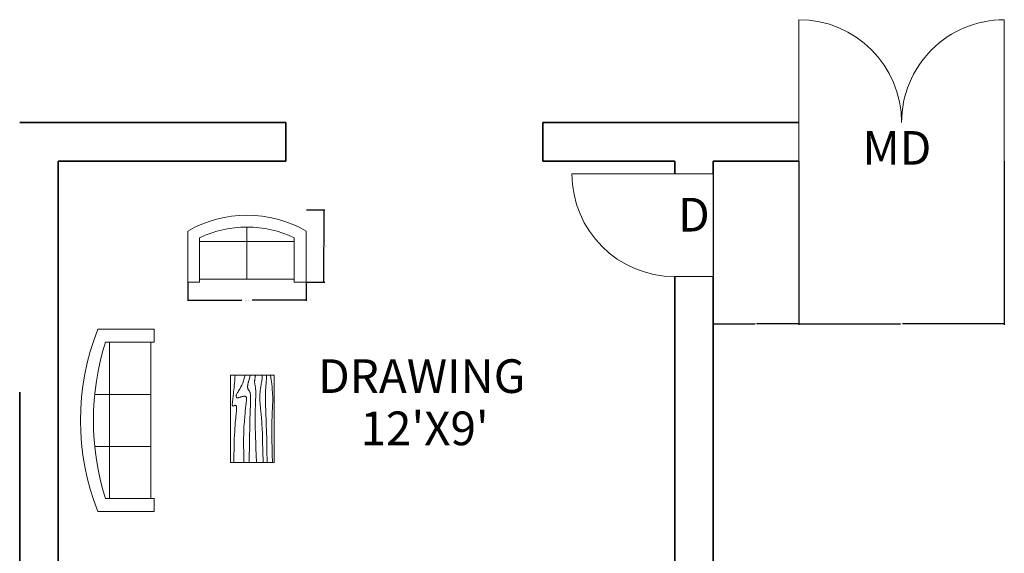
# Model space of a CAD drawing. Units: feet. Extents: x 2219 to 3039, y 1768 to 2369.
# Tile 5 of 16: x 2601 to 2831, y 2021 to 2146. Entities that reach past the tile are written whole.
import ezdxf

# ---------------------------------------------------------------- set-up
doc = ezdxf.new("R2010")
doc.units = ezdxf.units.FT
for name, color, linetype, lineweight in [('A-ANNO-DIMS', 2, 'Continuous', 18), ('A-ANNO-TEXT', 7, 'Continuous', 18), ('A-AREA-IDEN', 7, 'Continuous', 18), ('A-DOOR', 4, 'Continuous', 20), ('A-FURN', 8, 'Continuous', 18), ('A-WALL', 7, 'Continuous', 35)]:
    doc.layers.add(name, color=color, linetype=linetype, lineweight=lineweight)
doc.styles.get("Standard").update_dxf_attribs({"font": 'arial.ttf'})
doc.dimstyles.get("Standard").update_dxf_attribs({"dimtxt": 0.18, "dimasz": 0.18, "dimexe": 0.18, "dimexo": 0.0625, "dimgap": 0.09, "dimtad": 0, "dimtih": 1, "dimtoh": 1, "dimdec": 4, "dimzin": 0, "dimdsep": 46, "dimtxsty": 'Standard', "dimcen": 0.09, "dimadec": 0, "dimazin": 0, "dimtfac": 1, "dimtdec": 4, "dimtofl": 0, "dimtmove": 0, "dimatfit": 3, "dimfxl": 1, "dimtolj": 1, "dimtzin": 0, "dimarcsym": 0})

# ---------------------------------------------------------------- blocks, each defined once
blk = doc.blocks.new('Sofa - Roundback 7 ft.')
for p, q in [((-12.00002, -32.4421), (-12.00003, -6.5971)), ((11.99997, -32.4421), (11.99998, -6.5971)), ((-36.000027, -34), (-36.000027, -11.4696)), ((-35.999844, -13.3819), (35.9998, -13.3819)), ((35.99998, -34), (35.99998, -11.4696)), ((-36.000027, -32.4421), (35.99998, -32.4421))]:
    blk.add_line(p, q)
for points in [[(-36.000027, -34), (-42.000027, -34), (-42.000027, -8)], [(41.99998, -8), (41.99998, -34), (35.99998, -34)]]:
    blk.add_lwpolyline(points)
for centre, radius, start, end in [((0, -114.25), 114.25, 68.43141, 111.5686), ((-0.00001, -127.1968), 121.1968, 72.72033, 107.2797)]:
    blk.add_arc(centre, radius, start, end)
blk = doc.blocks.new('Sofa - Roundback Loveseat 5 ft.')
for p, q in [((0, -32.44198), (0, -5.99998)), ((-24, -33.99998), (-24, -11.46958)), ((-23.9998, -13.38178), (23.99986, -13.38178)), ((24.00004, -33.99998), (24.00004, -11.46958)), ((-24, -32.44198), (24.00004, -32.44198))]:
    blk.add_line(p, q)
for points in [[(-24, -33.99998), (-30, -33.99998), (-30, -7.99998)], [(30.00004, -7.99998), (30.00004, -33.99998), (24.00004, -33.99998)]]:
    blk.add_lwpolyline(points)
for centre, radius, start, end in [((0, -60.24998), 60.24998, 60.13715, 119.8628), ((0, -61.38438), 55.38444, 64.32083, 115.6792)]:
    blk.add_arc(centre, radius, start, end)
blk = doc.blocks.new('Table - Rectangular Woodgrain 60 x 30 in.')
for p, q in [((0, 0), (0, -30)), ((60, 0), (0, 0)), ((60, -30), (60, 0)), ((0, -30), (60, -30))]:
    blk.add_line(p, q)
for points in [[(0, -2.4), (4.8155, -2.418), (9.0302, -2.4688), (12.709, -2.5477), (15.9167, -2.65), (18.7181, -2.7711), (21.1781, -2.9063), (23.3616, -3.0508), (25.3333, -3.2), (27.1477, -3.3495), (28.8172, -3.4958), (30.3437, -3.636), (31.7291, -3.7667), (32.9756, -3.8849), (34.0849, -3.9875), (35.059, -4.0714), (35.9, -4.1334), (36.6114, -4.1711), (37.2041, -4.1854), (37.6906, -4.1779), (38.0833, -4.15), (38.3948, -4.1034), (38.6375, -4.0396), (38.8239, -3.9602), (38.9666, -3.8667), (39.0764, -3.7608), (39.1573, -3.6448), (39.2116, -3.521), (39.2416, -3.3917), (39.2498, -3.2593), (39.2385, -3.1261), (39.21, -2.9944), (39.1666, -2.8667), (39.111, -2.7447), (39.0468, -2.6281), (38.978, -2.5163), (38.9083, -2.4083), (38.8418, -2.3035), (38.7823, -2.201), (38.7337, -2.1001), (38.7, -2), (38.6844, -1.9003), (38.6875, -1.8021), (38.7094, -1.707), (38.75, -1.6167), (38.8094, -1.5326), (38.8875, -1.4563), (38.9844, -1.3893), (39.1, -1.3333), (39.2351, -1.2896), (39.3937, -1.2583), (39.5804, -1.2396), (39.8, -1.2333), (40.057, -1.2396), (40.3562, -1.2583), (40.7023, -1.2896), (41.1, -1.3333), (41.5547, -1.3895), (42.0755, -1.4573), (42.6721, -1.5361), (43.3542, -1.625), (44.1316, -1.7233), (45.014, -1.8302), (46.0114, -1.9449), (47.1333, -2.0667), (48.3862, -2.1947), (49.7625, -2.3281), (51.2513, -2.4663), (52.8416, -2.6083), (54.5226, -2.7535), (56.2833, -2.9011), (58.1127, -3.0501), (60, -3.2)], [(0, -9.2), (6.5759, -9.0858), (11.9385, -9.0365), (16.2527, -9.0418), (19.6833, -9.0917), (22.3952, -9.1759), (24.5531, -9.2844), (26.322, -9.4069), (27.8666, -9.5333), (29.3241, -9.6553), (30.7203, -9.7719), (32.0532, -9.8837), (33.3208, -9.9917), (34.5213, -10.0965), (35.6526, -10.199), (36.7128, -10.2999), (37.7, -10.4), (38.6129, -10.4996), (39.4531, -10.5969), (40.223, -10.6895), (40.925, -10.775), (41.5613, -10.8512), (42.1344, -10.9156), (42.6465, -10.966), (43.1, -11), (43.4976, -11.0158), (43.8437, -11.0136), (44.143, -10.9942), (44.4, -10.9583), (44.6195, -10.9069), (44.8062, -10.8406), (44.9648, -10.7603), (45.1, -10.6667), (45.2155, -10.5598), (45.3114, -10.4365), (45.3871, -10.2929), (45.4416, -10.125), (45.4743, -9.929), (45.4844, -9.7011), (45.4709, -9.4371), (45.4333, -9.1333), (45.3716, -8.7883), (45.2896, -8.4104), (45.1919, -8.0107), (45.0833, -7.6), (44.9685, -7.1893), (44.8521, -6.7896), (44.7388, -6.4117), (44.6333, -6.0667), (44.54, -5.7628), (44.4614, -5.4979), (44.4001, -5.2675), (44.3583, -5.0667), (44.3384, -4.8909), (44.3427, -4.7354), (44.3736, -4.5956), (44.4333, -4.4667), (44.5236, -4.3453), (44.6427, -4.2333), (44.7884, -4.1339), (44.9583, -4.05), (45.1501, -3.9849), (45.3614, -3.9417), (45.59, -3.9234), (45.8333, -3.9333), (46.0915, -3.9749), (46.3734, -4.0531), (46.6906, -4.1736), (47.0542, -4.3417), (47.4756, -4.5629), (47.9661, -4.8427), (48.5372, -5.1866), (49.2, -5.6), (49.9676, -6.0844), (50.8594, -6.625), (51.8965, -7.2031), (53.1, -7.8), (54.491, -8.3969), (56.0906, -8.975), (57.9199, -9.5156), (60, -10)], [(0, -12.8), (5.1847, -12.9322), (9.6213, -13.0323), (13.3963, -13.1059), (16.5958, -13.1583), (19.3063, -13.1952), (21.614, -13.2219), (23.6054, -13.2439), (25.3666, -13.2667), (26.9728, -13.2947), (28.4531, -13.3281), (29.8256, -13.3663), (31.1083, -13.4083), (32.3191, -13.4535), (33.476, -13.501), (34.597, -13.5501), (35.7, -13.6), (36.7984, -13.6497), (37.8875, -13.6979), (38.9578, -13.743), (40, -13.7833), (41.0047, -13.8174), (41.9625, -13.8438), (42.864, -13.8607), (43.7, -13.8667), (44.4631, -13.8604), (45.1552, -13.8417), (45.7801, -13.8104), (46.3416, -13.7667), (46.8439, -13.7104), (47.2906, -13.6417), (47.6858, -13.5604), (48.0333, -13.4667), (48.3375, -13.3608), (48.6042, -13.2448), (48.8396, -13.121), (49.05, -12.9917), (49.2417, -12.8593), (49.4208, -12.7261), (49.5937, -12.5944), (49.7667, -12.4667), (49.9452, -12.3451), (50.1323, -12.2313), (50.3303, -12.1268), (50.5416, -12.0333), (50.7686, -11.9524), (51.0135, -11.8854), (51.2788, -11.8341), (51.5666, -11.8), (51.8785, -11.7843), (52.2116, -11.7865), (52.562, -11.8059), (52.926, -11.8417), (53.2998, -11.8931), (53.6795, -11.9594), (54.0614, -12.0397), (54.4416, -12.1333), (54.8223, -12.2401), (55.2293, -12.3625), (55.6942, -12.5037), (56.2489, -12.6667), (56.9251, -12.8547), (57.7545, -13.0708), (58.7689, -13.3182), (60, -13.6)], [(0, -18), (5.124, -17.7273), (9.6609, -17.5057), (13.6705, -17.3303), (17.2125, -17.1958), (20.3467, -17.0973), (23.1328, -17.0297), (25.6307, -16.9878), (27.9, -16.9667), (29.9928, -16.9617), (31.9302, -16.9703), (33.7254, -16.9907), (35.3917, -17.0208), (36.9423, -17.0588), (38.3906, -17.1026), (39.7499, -17.1503), (41.0333, -17.2), (42.2519, -17.2496), (43.4073, -17.2969), (44.4986, -17.3395), (45.525, -17.375), (46.4858, -17.4012), (47.3802, -17.4156), (48.2074, -17.416), (48.9667, -17.4), (49.6583, -17.3662), (50.2872, -17.3167), (50.8595, -17.2547), (51.3812, -17.1833), (51.8584, -17.1057), (52.2971, -17.025), (52.7034, -16.9443), (53.0833, -16.8667), (53.443, -16.7951), (53.789, -16.7313), (54.128, -16.6768), (54.4666, -16.6334), (54.8115, -16.6024), (55.1693, -16.5854), (55.5465, -16.5841), (55.95, -16.6), (56.3828, -16.6337), (56.8346, -16.6823), (57.2915, -16.7418), (57.7396, -16.8084), (58.165, -16.878), (58.5539, -16.9469), (58.8924, -17.0111), (59.1666, -17.0667), (59.3679, -17.1107), (59.5078, -17.1438), (59.6032, -17.1675), (59.6708, -17.1833), (59.7275, -17.193), (59.7901, -17.1979), (59.8753, -17.1998), (60, -17.2)], [(0, -22.4), (8.0098, -22.2501), (14.4094, -22.1011), (19.4168, -21.9535), (23.25, -21.8083), (26.1269, -21.6663), (28.2656, -21.5281), (29.884, -21.3947), (31.2, -21.2667), (32.3967, -21.1448), (33.5172, -21.0292), (34.5697, -20.9198), (35.5625, -20.8167), (36.5037, -20.7198), (37.4015, -20.6292), (38.2642, -20.5448), (39.1, -20.4667), (39.9164, -20.3951), (40.7187, -20.3313), (41.5117, -20.2768), (42.3, -20.2333), (43.0883, -20.2024), (43.8812, -20.1854), (44.6836, -20.1841), (45.5, -20.2), (46.3328, -20.234), (47.1747, -20.2844), (48.0163, -20.3488), (48.8479, -20.425), (49.66, -20.5106), (50.4429, -20.6031), (51.1872, -20.7004), (51.8833, -20.8), (52.5246, -20.8999), (53.1166, -20.9995), (53.6681, -21.0983), (54.1875, -21.1958), (54.6834, -21.2919), (55.1646, -21.3859), (55.6394, -21.4777), (56.1167, -21.5667), (56.6028, -21.6515), (57.0961, -21.7266), (57.5929, -21.7852), (58.0896, -21.8208), (58.5823, -21.8268), (59.0674, -21.7964), (59.5412, -21.723), (60, -21.6)], [(0, -25.2), (8.6355, -25.0504), (15.7026, -24.9031), (21.4049, -24.7606), (25.9458, -24.625), (29.529, -24.4988), (32.3578, -24.3844), (34.6359, -24.284), (36.5667, -24.2), (38.3213, -24.1341), (39.9417, -24.0854), (41.437, -24.0523), (42.8167, -24.0333), (44.0901, -24.0268), (45.2667, -24.0313), (46.3557, -24.0451), (47.3667, -24.0667), (48.309, -24.0947), (49.1928, -24.1287), (50.0284, -24.168), (50.826, -24.2125), (51.5959, -24.2617), (52.3483, -24.3151), (53.0935, -24.3725), (53.8417, -24.4334), (54.6009, -24.497), (55.3699, -24.561), (56.1454, -24.6226), (56.9239, -24.6792), (57.7021, -24.7279), (58.4764, -24.7662), (59.2435, -24.7911), (60, -24.8)], [(0, -28.8), (5.6867, -28.6681), (10.45, -28.5698), (14.407, -28.5012), (17.675, -28.4584), (20.3711, -28.4374), (22.6125, -28.4344), (24.5164, -28.4455), (26.2, -28.4667), (27.762, -28.4947), (29.2276, -28.5281), (30.6033, -28.5663), (31.8958, -28.6084), (33.1118, -28.6535), (34.2578, -28.7011), (35.3405, -28.7501), (36.3666, -28.8), (37.3443, -28.8497), (38.288, -28.8974), (39.2137, -28.9412), (40.1375, -28.9792), (41.0753, -29.0093), (42.0432, -29.0297), (43.0572, -29.0384), (44.1333, -29.0333), (45.2936, -29.0114), (46.5843, -28.9641), (48.0579, -28.8816), (49.7666, -28.7542), (51.7629, -28.5721), (54.0989, -28.3255), (56.8272, -28.0048), (60, -27.6)]]:
    blk.add_lwpolyline(points)
blk = doc.blocks.new('DOOR-24-LEAF')
blk.add_line((33, 0), (0, 0))
blk.add_arc((9, 0), 24, 0, 90)
blk = doc.blocks.new('DOOR-24-INTEGRAL-JAMB')
for p, q in [((9, 24), (0, 24)), ((33, 0), (0, 0))]:
    blk.add_line(p, q)
blk.add_arc((9, 0), 24, 0, 90)
blk = doc.blocks.new('*D26')
at = {"layer": 'A-ANNO-DIMS', "color": 0, "lineweight": -2, "transparency": 16777216}
for p, q in [((2640.66, 2084.53), (2640.66, 2080.26)), ((2668.31, 2084.53), (2668.31, 2080.26)), ((2640.84, 2080.44), (2653.26, 2080.44)), ((2668.13, 2080.44), (2655.71, 2080.44))]:
    blk.add_line(p, q, dxfattribs=at)
at = {"layer": 'A-ANNO-DIMS', "color": 0, "transparency": 16777216}
for points in [[(2640.84, 2080.47), (2640.84, 2080.41), (2640.66, 2080.44)], [(2668.13, 2080.47), (2668.13, 2080.41), (2668.31, 2080.44)]]:
    blk.add_solid(points, dxfattribs=at)
at = {"layer": 'Defpoints', "color": 0, "transparency": 16777216}
for p in [(2640.66, 2084.59), (2668.31, 2084.59), (2668.31, 2080.44)]:
    blk.add_point(p, dxfattribs=at)
at = {"layer": 'A-ANNO-DIMS', "color": 0, "transparency": 16777216, "insert": (2654.49, 2080.44), "char_height": 0.18, "attachment_point": 5}
blk.add_mtext('\\A1;LOVESEAT 28 TYP.', dxfattribs=at)
blk = doc.blocks.new('*D27')
at = {"layer": 'A-ANNO-DIMS', "color": 0, "lineweight": -2, "transparency": 16777216}
for p, q in [((2668.38, 2101.49), (2672.64, 2101.49)), ((2672.46, 2101.31), (2672.46, 2093.22)), ((2672.46, 2084.77), (2672.46, 2092.86)), ((2668.38, 2084.59), (2672.64, 2084.59))]:
    blk.add_line(p, q, dxfattribs=at)
at = {"layer": 'A-ANNO-DIMS', "color": 0, "transparency": 16777216}
for points in [[(2672.43, 2101.31), (2672.49, 2101.31), (2672.46, 2101.49)], [(2672.43, 2084.77), (2672.49, 2084.77), (2672.46, 2084.59)]]:
    blk.add_solid(points, dxfattribs=at)
at = {"layer": 'Defpoints', "color": 0, "transparency": 16777216}
for p in [(2668.31, 2101.49), (2672.46, 2101.49), (2668.31, 2084.59)]:
    blk.add_point(p, dxfattribs=at)
at = {"layer": 'A-ANNO-DIMS', "color": 0, "transparency": 16777216, "insert": (2672.46, 2093.04), "char_height": 0.18, "attachment_point": 5}
blk.add_mtext('\\A1;17 TYP.', dxfattribs=at)
blk = doc.blocks.new('*D59')
at = {"layer": 'A-ANNO-DIMS', "color": 0, "lineweight": -2, "transparency": 16777216}
for p, q in [((2763.4, 2112.86), (2763.4, 2074.69)), ((2783.4, 2112.86), (2783.4, 2074.69)), ((2763.58, 2074.87), (2773.18, 2074.87)), ((2783.22, 2074.87), (2773.62, 2074.87))]:
    blk.add_line(p, q, dxfattribs=at)
at = {"layer": 'A-ANNO-DIMS', "color": 0, "transparency": 16777216}
for points in [[(2763.58, 2074.9), (2763.58, 2074.84), (2763.4, 2074.87)], [(2783.22, 2074.9), (2783.22, 2074.84), (2783.4, 2074.87)]]:
    blk.add_solid(points, dxfattribs=at)
at = {"layer": 'Defpoints', "color": 0, "transparency": 16777216}
for p in [(2763.4, 2112.92), (2783.4, 2112.92), (2763.4, 2074.87)]:
    blk.add_point(p, dxfattribs=at)
at = {"layer": 'A-ANNO-DIMS', "color": 0, "transparency": 16777216, "insert": (2773.4, 2074.87), "char_height": 0.18, "attachment_point": 5}
blk.add_mtext('\\A1;20', dxfattribs=at)
blk = doc.blocks.new('*D60')
at = {"layer": 'A-ANNO-DIMS', "color": 0, "lineweight": -2, "transparency": 16777216}
for p, q in [((2783.4, 2112.86), (2783.4, 2074.69)), ((2831.4, 2112.86), (2831.4, 2074.69)), ((2783.58, 2074.87), (2807.18, 2074.87)), ((2831.22, 2074.87), (2807.62, 2074.87))]:
    blk.add_line(p, q, dxfattribs=at)
at = {"layer": 'A-ANNO-DIMS', "color": 0, "transparency": 16777216}
for points in [[(2783.58, 2074.9), (2783.58, 2074.84), (2783.4, 2074.87)], [(2831.22, 2074.9), (2831.22, 2074.84), (2831.4, 2074.87)]]:
    blk.add_solid(points, dxfattribs=at)
at = {"layer": 'Defpoints', "color": 0, "transparency": 16777216}
for p in [(2783.4, 2112.92), (2831.4, 2112.92), (2783.4, 2074.87)]:
    blk.add_point(p, dxfattribs=at)
at = {"layer": 'A-ANNO-DIMS', "color": 0, "transparency": 16777216, "insert": (2807.4, 2074.87), "char_height": 0.18, "attachment_point": 5}
blk.add_mtext('\\A1;48', dxfattribs=at)

msp = doc.modelspace()

# ---------------------------------------------------------------- linework, layer by layer
at = {"layer": 'A-WALL'}
for p, q in [((2663.585, 2121.923), (2601.4, 2121.923)), ((2663.585, 2121.923), (2663.585, 2112.923)), ((2723.585, 2112.923), (2723.585, 2121.923)), ((2783.4, 2121.923), (2723.585, 2121.923)), ((2610.4, 2112.923), (2663.585, 2112.923)), ((2610.4, 2004.923), (2610.4, 2112.923)), ((2723.585, 2112.923), (2754.4, 2112.923)), ((2754.4, 2112.923), (2754.4, 2109.923)), ((2763.4, 2112.923), (2763.4, 2109.923)), ((2783.4, 2112.923), (2763.4, 2112.923)), ((2754.4, 2085.923), (2754.4, 2004.923)), ((2763.4, 2085.923), (2763.4, 1995.923)), ((2601.4, 1906.923), (2601.4, 2058.923))]:
    msp.add_line(p, q, dxfattribs=at)

# ---------------------------------------------------------------- block references
at = {"layer": 'A-DOOR', "extrusion": (0, 0, -1), "zscale": -1, "rotation": 90.00000000000047}
msp.add_blockref('DOOR-24-LEAF', (-2783.4, 2112.923), dxfattribs=at)
at = {"layer": 'A-DOOR'}
for name, p, rotation in [('DOOR-24-LEAF', (2831.399, 2112.923), 89.99999999999905), ('DOOR-24-INTEGRAL-JAMB', (2763.399, 2109.922), 180)]:
    msp.add_blockref(name, p, dxfattribs=dict(at, rotation=rotation))
at = {"layer": 'A-FURN', "xscale": 0.4609193945856732, "yscale": 0.4609193945856732, "zscale": 0.4609193945856732}
msp.add_blockref('Sofa - Roundback Loveseat 5 ft.', (2654.486, 2100.263), dxfattribs=at)
at = {"layer": 'A-FURN', "rotation": 90}
for name, p, xscale, yscale, zscale in [('Sofa - Roundback 7 ft.', (2615.597, 2052.346), 0.5063942958922181, 0.5063942958922181, 0.5063942958922181), ('Table - Rectangular Woodgrain 60 x 30 in.', (2650.633, 2042.527), 0.3400232329989347, 0.3400232329989347, 0.3400232329989347)]:
    msp.add_blockref(name, p, dxfattribs=dict(at, xscale=xscale, yscale=yscale, zscale=zscale))

# ---------------------------------------------------------------- texts
at = {"layer": 'A-ANNO-TEXT'}
for s, height, p in [('MD', 7.8584, (2798.279, 2112.061)), ('D', 7.858, (2755.211, 2096.446))]:
    msp.add_text(s, height=height, dxfattribs=at).set_placement(p)
at = {"layer": 'A-AREA-IDEN'}
for s, p in [('DRAWING', (2671.123, 2058.752)), ("12'X9'", (2681.007, 2046.558))]:
    msp.add_text(s, height=7.8584, dxfattribs=at).set_placement(p)

# ---------------------------------------------------------------- dimensions: what is measured, and where the dimension line sits
at = {"layer": 'A-ANNO-DIMS'}
for base, p1, p2, picture, middle in [((2763.4, 2074.873), (2783.4, 2112.923), (2763.4, 2112.923), '*D59', (2773.4, 2074.873)), ((2783.4, 2074.873), (2831.4, 2112.923), (2783.4, 2112.923), '*D60', (2807.4, 2074.873))]:
    dim = msp.add_linear_dim(base=base, p1=p1, p2=p2, angle=180, dimstyle='Standard', override={"dimdec": 0, "dimlfac": 1, "dimrnd": 0, "dimzin": 0, "dimdsep": 46, "dimlunit": 2}, dxfattribs=at)
    dim.commit()
    dim.dimension.update_dxf_attribs({"geometry": picture, "text_midpoint": middle})
dim = msp.add_linear_dim(base=(2672.462, 2101.492), p1=(2668.313, 2084.592), p2=(2668.313, 2101.492), angle=90, text='<> TYP.', dimstyle='Standard', override={"dimdec": 0, "dimlfac": 1, "dimrnd": 0, "dimzin": 0, "dimdsep": 46, "dimlunit": 2}, dxfattribs=at)
dim.commit()
dim.dimension.update_dxf_attribs({"geometry": '*D27', "text_midpoint": (2672.462, 2093.042)})
dim = msp.add_linear_dim(base=(2668.313, 2080.443), p1=(2640.658, 2084.592), p2=(2668.313, 2084.592), text='LOVESEAT <> TYP.', dimstyle='Standard', override={"dimdec": 0, "dimlfac": 1, "dimrnd": 0, "dimzin": 0, "dimdsep": 46, "dimlunit": 2}, dxfattribs=at)
dim.commit()
dim.dimension.update_dxf_attribs({"geometry": '*D26', "text_midpoint": (2654.486, 2080.443)})

doc.saveas('drawing.dxf')
